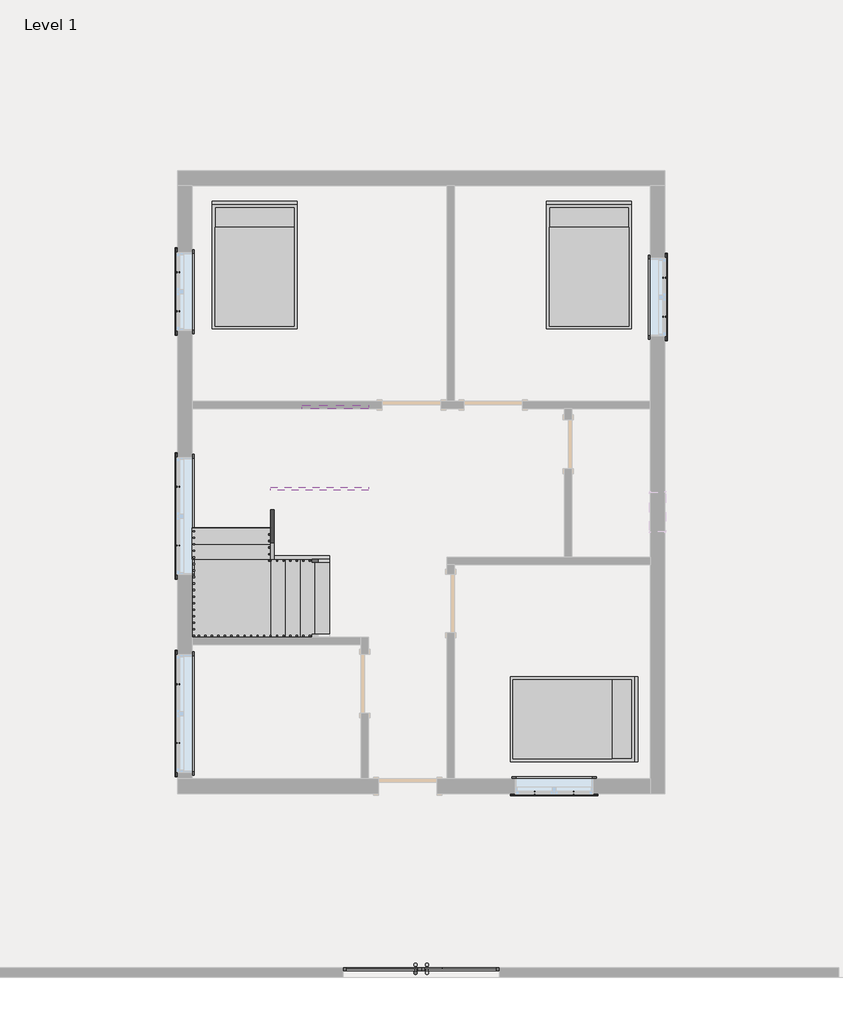
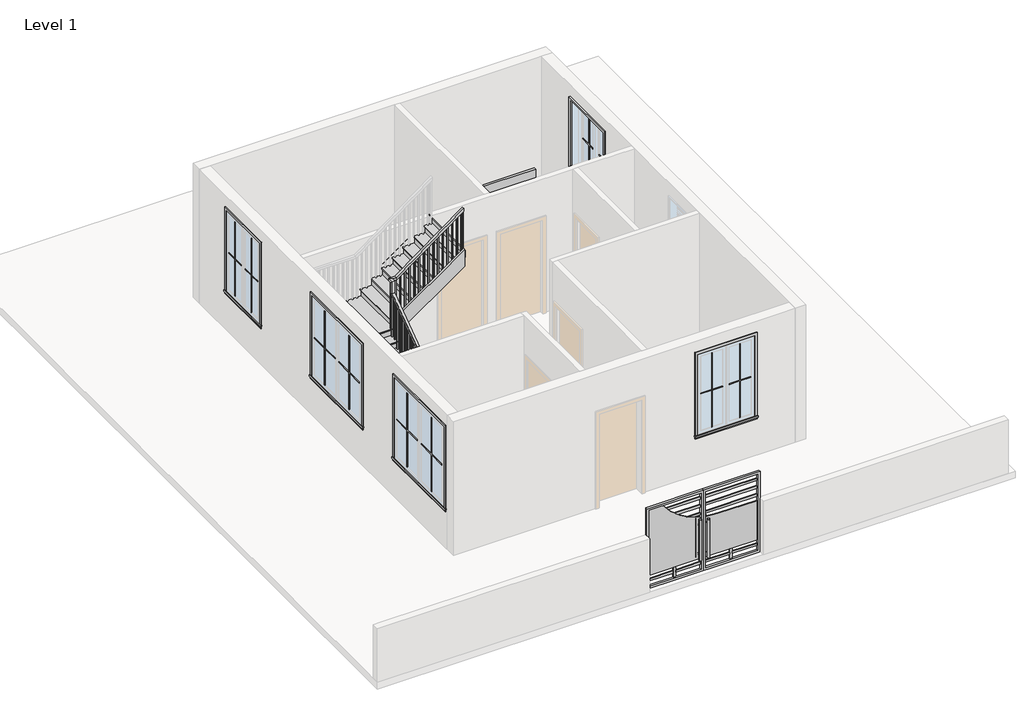
# One storey, part 3 of 3: 21 proxies, 5 members, 3 furniture elements, 1 railing, 1 stair flight.
"""IFC4 building model written with IfcOpenShell, lengths in millimetres."""

from ifc_helpers import new_model, si_unit, frame, origin, place, context, project, spatial, polyline, outline, extrude, faceted_brep, transform, mapped, element, save
from components import generic_models_113f6068, muntin_pattern_2x2_muntin_pattern_2x2_0a037076, muntin_pattern_2x2_muntin_pattern_2x2_e6f69628, muntin_pattern_2x2_muntin_pattern_2x2_2b4d9f72, muntin_pattern_2x2_muntin_pattern_2x2_ef995ed3, trim_window_exterior_flat_with_sill_b601e94a, trim_window_exterior_flat_with_sill_b7e4d11c, trim_window_interior_flat_picture_frame_bfefb25c, trim_window_interior_flat_picture_frame_936b8d2a, bed_17739_bed_17739_15c61121, stair_flight_0ad16ec4

model = new_model("IFC4")

# Units and contexts
model_context = context("Model", 3, world=origin())
ifc_project = project(units=[si_unit("LENGTHUNIT", "METRE", prefix="MILLI")], contexts=[model_context])

# Site, building, storey
site = spatial("IfcSite", under=ifc_project)
building = spatial("IfcBuilding", under=site)
storey = spatial("IfcBuildingStorey", under=building, Name="Level 1", Elevation=0.0)

# Proxies
placement = place(None, origin())
generic_models_shape = generic_models_113f6068(model_context)
element("IfcBuildingElementProxy", 1, Name="Generic Models", at=placement, inside=storey, context=model_context, shape_type="MappedRepresentation", body=[
    mapped(generic_models_shape, transform((-1254.3605391, -7873.6106437, 0.0), x_axis=(1.0, 0.0, 0.0), y_axis=(0.0, 1.0, 0.0), z_axis=(0.0, 0.0, 1.0))),
])
muntin_pattern_2x2_muntin_pattern_2x2_shape = muntin_pattern_2x2_muntin_pattern_2x2_0a037076(model_context)
element("IfcBuildingElementProxy", 2, Name="Muntin Pattern_2x2 : Muntin Pattern_2x2", ObjectType="Muntin Pattern_2x2 : Muntin Pattern_2x2", at=placement, inside=storey, context=model_context, shape_type="MappedRepresentation", body=[
    mapped(muntin_pattern_2x2_muntin_pattern_2x2_shape, transform((-5035.7855391, -4380.9248761, 984.25), x_axis=(0.0, 1.0, 0.0), y_axis=(-1.0, 0.0, 0.0), z_axis=(0.0, 0.0, 1.0))),
])
element("IfcBuildingElementProxy", 3, Name="Muntin Pattern_2x2 : Muntin Pattern_2x2", ObjectType="Muntin Pattern_2x2 : Muntin Pattern_2x2", at=placement, inside=storey, context=model_context, shape_type="MappedRepresentation", body=[
    mapped(muntin_pattern_2x2_muntin_pattern_2x2_shape, transform((-5035.7855391, -1310.6998761, 984.25), x_axis=(0.0, 1.0, 0.0), y_axis=(-1.0, 0.0, 0.0), z_axis=(0.0, 0.0, 1.0))),
])
muntin_pattern_2x2_muntin_pattern_2x2_2_shape = muntin_pattern_2x2_muntin_pattern_2x2_e6f69628(model_context)
element("IfcBuildingElementProxy", 4, Name="Muntin Pattern_2x2 : Muntin Pattern_2x2", ObjectType="Muntin Pattern_2x2 : Muntin Pattern_2x2", at=placement, inside=storey, context=model_context, shape_type="MappedRepresentation", body=[
    mapped(muntin_pattern_2x2_muntin_pattern_2x2_2_shape, transform((-5035.7855391, -3469.6998761, 984.25), x_axis=(0.0, -1.0, 0.0), y_axis=(1.0, 0.0, 0.0), z_axis=(0.0, 0.0, 1.0))),
])
element("IfcBuildingElementProxy", 5, Name="Muntin Pattern_2x2 : Muntin Pattern_2x2", ObjectType="Muntin Pattern_2x2 : Muntin Pattern_2x2", at=placement, inside=storey, context=model_context, shape_type="MappedRepresentation", body=[
    mapped(muntin_pattern_2x2_muntin_pattern_2x2_2_shape, transform((-5035.7855391, -399.4748761, 984.25), x_axis=(0.0, -1.0, 0.0), y_axis=(1.0, 0.0, 0.0), z_axis=(0.0, 0.0, 1.0))),
])
muntin_pattern_2x2_muntin_pattern_2x2_3_shape = muntin_pattern_2x2_muntin_pattern_2x2_2b4d9f72(model_context)
element("IfcBuildingElementProxy", 6, Name="Muntin Pattern_2x2 : Muntin Pattern_2x2", ObjectType="Muntin Pattern_2x2 : Muntin Pattern_2x2", at=placement, inside=storey, context=model_context, shape_type="MappedRepresentation", body=[
    mapped(muntin_pattern_2x2_muntin_pattern_2x2_3_shape, transform((1115.7769609, -5157.2123761, 984.25), x_axis=(-1.0, 0.0, 0.0), y_axis=(0.0, -1.0, 0.0), z_axis=(0.0, 0.0, 1.0))),
])
element("IfcBuildingElementProxy", 7, Name="Muntin Pattern_2x2 : Muntin Pattern_2x2", ObjectType="Muntin Pattern_2x2 : Muntin Pattern_2x2", at=placement, inside=storey, context=model_context, shape_type="MappedRepresentation", body=[
    mapped(muntin_pattern_2x2_muntin_pattern_2x2_3_shape, transform((2527.0644609, 2851.7251239, 984.25), x_axis=(0.0, -1.0, 0.0), y_axis=(1.0, 0.0, 0.0), z_axis=(0.0, 0.0, 1.0))),
])
element("IfcBuildingElementProxy", 8, Name="Muntin Pattern_2x2 : Muntin Pattern_2x2", ObjectType="Muntin Pattern_2x2 : Muntin Pattern_2x2", at=placement, inside=storey, context=model_context, shape_type="MappedRepresentation", body=[
    mapped(muntin_pattern_2x2_muntin_pattern_2x2_3_shape, transform((-5035.7855391, 2331.0251239, 984.25), x_axis=(0.0, 1.0, 0.0), y_axis=(-1.0, 0.0, 0.0), z_axis=(0.0, 0.0, 1.0))),
])
muntin_pattern_2x2_muntin_pattern_2x2_4_shape = muntin_pattern_2x2_muntin_pattern_2x2_ef995ed3(model_context)
element("IfcBuildingElementProxy", 9, Name="Muntin Pattern_2x2 : Muntin Pattern_2x2", ObjectType="Muntin Pattern_2x2 : Muntin Pattern_2x2", at=placement, inside=storey, context=model_context, shape_type="MappedRepresentation", body=[
    mapped(muntin_pattern_2x2_muntin_pattern_2x2_4_shape, transform((509.3519609, -5157.2123761, 984.25), x_axis=(1.0, 0.0, 0.0), y_axis=(0.0, 1.0, 0.0), z_axis=(0.0, 0.0, 1.0))),
])
element("IfcBuildingElementProxy", 10, Name="Muntin Pattern_2x2 : Muntin Pattern_2x2", ObjectType="Muntin Pattern_2x2 : Muntin Pattern_2x2", at=placement, inside=storey, context=model_context, shape_type="MappedRepresentation", body=[
    mapped(muntin_pattern_2x2_muntin_pattern_2x2_4_shape, transform((2527.0644609, 2245.3001239, 984.25), x_axis=(0.0, 1.0, 0.0), y_axis=(-1.0, 0.0, 0.0), z_axis=(0.0, 0.0, 1.0))),
])
element("IfcBuildingElementProxy", 11, Name="Muntin Pattern_2x2 : Muntin Pattern_2x2", ObjectType="Muntin Pattern_2x2 : Muntin Pattern_2x2", at=placement, inside=storey, context=model_context, shape_type="MappedRepresentation", body=[
    mapped(muntin_pattern_2x2_muntin_pattern_2x2_4_shape, transform((-5035.7855391, 2937.4501239, 984.25), x_axis=(0.0, -1.0, 0.0), y_axis=(1.0, 0.0, 0.0), z_axis=(0.0, 0.0, 1.0))),
])
trim_window_exterior_flat_with_sill_shape = trim_window_exterior_flat_with_sill_b601e94a(model_context)
element("IfcBuildingElementProxy", 12, Name="Trim-Window-Exterior-Flat : with Sill", ObjectType="Trim-Window-Exterior-Flat : with Sill", at=placement, inside=storey, context=model_context, shape_type="MappedRepresentation", body=[
    mapped(trim_window_exterior_flat_with_sill_shape, transform((-5045.3105391, -3925.3123761, 2743.2), x_axis=(0.0, -1.0, 0.0), y_axis=(0.0, 0.0, 1.0), z_axis=(-1.0, 0.0, 0.0))),
])
element("IfcBuildingElementProxy", 13, Name="Trim-Window-Exterior-Flat : with Sill", ObjectType="Trim-Window-Exterior-Flat : with Sill", at=placement, inside=storey, context=model_context, shape_type="MappedRepresentation", body=[
    mapped(trim_window_exterior_flat_with_sill_shape, transform((-5045.3105391, -855.0873761, 2743.2), x_axis=(0.0, -1.0, 0.0), y_axis=(0.0, 0.0, 1.0), z_axis=(-1.0, 0.0, 0.0))),
])
trim_window_exterior_flat_with_sill_2_shape = trim_window_exterior_flat_with_sill_b7e4d11c(model_context)
element("IfcBuildingElementProxy", 14, Name="Trim-Window-Exterior-Flat : with Sill", ObjectType="Trim-Window-Exterior-Flat : with Sill", at=placement, inside=storey, context=model_context, shape_type="MappedRepresentation", body=[
    mapped(trim_window_exterior_flat_with_sill_2_shape, transform((812.5644609, -5166.7373761, 2743.2), x_axis=(1.0, 0.0, 0.0), y_axis=(0.0, 0.0, 1.0), z_axis=(0.0, -1.0, 0.0))),
])
element("IfcBuildingElementProxy", 15, Name="Trim-Window-Exterior-Flat : with Sill", ObjectType="Trim-Window-Exterior-Flat : with Sill", at=placement, inside=storey, context=model_context, shape_type="MappedRepresentation", body=[
    mapped(trim_window_exterior_flat_with_sill_2_shape, transform((2536.5894609, 2548.5126239, 2743.2), x_axis=(0.0, 1.0, 0.0), y_axis=(0.0, 0.0, 1.0), z_axis=(1.0, 0.0, 0.0))),
])
element("IfcBuildingElementProxy", 16, Name="Trim-Window-Exterior-Flat : with Sill", ObjectType="Trim-Window-Exterior-Flat : with Sill", at=placement, inside=storey, context=model_context, shape_type="MappedRepresentation", body=[
    mapped(trim_window_exterior_flat_with_sill_2_shape, transform((-5045.3105391, 2634.2376239, 2743.2), x_axis=(0.0, -1.0, 0.0), y_axis=(0.0, 0.0, 1.0), z_axis=(-1.0, 0.0, 0.0))),
])
trim_window_interior_flat_picture_frame_shape = trim_window_interior_flat_picture_frame_bfefb25c(model_context)
element("IfcBuildingElementProxy", 17, Name="Trim-Window-Interior-Flat : Picture Frame", ObjectType="Trim-Window-Interior-Flat : Picture Frame", at=placement, inside=storey, context=model_context, shape_type="MappedRepresentation", body=[
    mapped(trim_window_interior_flat_picture_frame_shape, transform((-4816.7105391, -3925.3123761, 2743.2), x_axis=(0.0, 1.0, 0.0), y_axis=(0.0, 0.0, 1.0), z_axis=(1.0, 0.0, 0.0))),
])
element("IfcBuildingElementProxy", 18, Name="Trim-Window-Interior-Flat : Picture Frame", ObjectType="Trim-Window-Interior-Flat : Picture Frame", at=placement, inside=storey, context=model_context, shape_type="MappedRepresentation", body=[
    mapped(trim_window_interior_flat_picture_frame_shape, transform((-4816.7105391, -855.0873761, 2743.2), x_axis=(0.0, 1.0, 0.0), y_axis=(0.0, 0.0, 1.0), z_axis=(1.0, 0.0, 0.0))),
])
trim_window_interior_flat_picture_frame_2_shape = trim_window_interior_flat_picture_frame_936b8d2a(model_context)
element("IfcBuildingElementProxy", 19, Name="Trim-Window-Interior-Flat : Picture Frame", ObjectType="Trim-Window-Interior-Flat : Picture Frame", at=placement, inside=storey, context=model_context, shape_type="MappedRepresentation", body=[
    mapped(trim_window_interior_flat_picture_frame_2_shape, transform((812.5644609, -4938.1373761, 2743.2), x_axis=(-1.0, 0.0, 0.0), y_axis=(0.0, 0.0, 1.0), z_axis=(0.0, 1.0, 0.0))),
])
element("IfcBuildingElementProxy", 20, Name="Trim-Window-Interior-Flat : Picture Frame", ObjectType="Trim-Window-Interior-Flat : Picture Frame", at=placement, inside=storey, context=model_context, shape_type="MappedRepresentation", body=[
    mapped(trim_window_interior_flat_picture_frame_2_shape, transform((2307.9894609, 2548.5126239, 2743.2), x_axis=(0.0, -1.0, 0.0), y_axis=(0.0, 0.0, 1.0), z_axis=(-1.0, 0.0, 0.0))),
])
element("IfcBuildingElementProxy", 21, Name="Trim-Window-Interior-Flat : Picture Frame", ObjectType="Trim-Window-Interior-Flat : Picture Frame", at=placement, inside=storey, context=model_context, shape_type="MappedRepresentation", body=[
    mapped(trim_window_interior_flat_picture_frame_2_shape, transform((-4816.7105391, 2634.2376239, 2743.2), x_axis=(0.0, 1.0, 0.0), y_axis=(0.0, 0.0, 1.0), z_axis=(1.0, 0.0, 0.0))),
])

# Furniture
bed_17739_bed_17739_shape = bed_17739_bed_17739_15c61121(model_context)
element("IfcFurniture", 22, ObjectType="Bed_17739 : Bed_17739", at=placement, inside=storey, context=model_context, shape_type="MappedRepresentation", body=[
    mapped(bed_17739_bed_17739_shape, transform((-3845.1605391, 3024.7626239, 0.0), x_axis=(1.0, 0.0, 0.0), y_axis=(0.0, 1.0, 0.0), z_axis=(0.0, 0.0, 1.0))),
])
element("IfcFurniture", 23, ObjectType="Bed_17739 : Bed_17739", at=placement, inside=storey, context=model_context, shape_type="MappedRepresentation", body=[
    mapped(bed_17739_bed_17739_shape, transform((1355.4894609, 3024.7626239, 0.0), x_axis=(1.0, 0.0, 0.0), y_axis=(0.0, 1.0, 0.0), z_axis=(0.0, 0.0, 1.0))),
])
element("IfcFurniture", 24, ObjectType="Bed_17739 : Bed_17739", at=placement, inside=storey, context=model_context, shape_type="MappedRepresentation", body=[
    mapped(bed_17739_bed_17739_shape, transform((1101.4894609, -4011.0373761, 0.0), x_axis=(0.0, -1.0, 0.0), y_axis=(1.0, 0.0, 0.0), z_axis=(0.0, 0.0, 1.0))),
])

# Members
element("IfcMember", 25, ObjectType="Stringer - 2\" Width", at=placement, inside=storey, context=model_context, shape_type="SweptSolid", body=[
    extrude(outline(polyline([(0.0, -2683.1105391), (150.5087903, -2683.1105391), (150.5087903, -3112.2707489), (0.0, -2897.7957228), (0.0, -2683.1105391)])), frame((0.0, -2791.8373761, 0.0), z_axis=(0.0, 1.0, 0.0), x_axis=(0.0, 0.0, 1.0)), (0.0, 0.0, 1.0), 50.8),
])
element("IfcMember", 26, ObjectType="Stringer - 2\" Width", at=placement, inside=storey, context=model_context, shape_type="SweptSolid", body=[
    extrude(outline(polyline([(2327.4856495, -2580.7583047), (2683.4489938, -2073.5105391), (3055.8117181, -2073.5105391), (2327.4856495, -3111.3751869), (2327.4856495, -2580.7583047)])), frame((0.0, 814.9626239, 0.0), z_axis=(0.0, 1.0, 0.0), x_axis=(0.0, 0.0, 1.0)), (0.0, 0.0, 1.0), 50.8),
])
element("IfcMember", 27, ObjectType="Stringer - 2\" Width", at=placement, inside=storey, context=model_context, shape_type="SweptSolid", body=[
    extrude(outline(polyline([(0.0, -2683.1105391), (221.706455, -2683.1105391), (827.7415427, -3546.7105391), (455.3788184, -3546.7105391), (0.0, -2897.7957228), (0.0, -2683.1105391)])), frame((0.0, -1521.8373761, 0.0), z_axis=(0.0, 1.0, 0.0), x_axis=(0.0, 0.0, 1.0)), (0.0, 0.0, 1.0), 50.8),
])
element("IfcMember", 28, ObjectType="Stringer - 2\" Width", at=placement, inside=storey, context=model_context, shape_type="SweptSolid", body=[
    extrude(outline(polyline([(-1521.8373761, 650.3564629), (-1521.8373761, 1025.5327137), (-455.0373761, 1791.1786467), (-455.0373761, 1416.0023959), (-1521.8373761, 650.3564629)])), frame((-3597.5105391, 0.0, 0.0), z_axis=(1.0, 0.0, 0.0), x_axis=(0.0, 1.0, 0.0)), (0.0, 0.0, 1.0), 50.8),
])
element("IfcMember", 29, ObjectType="Stringer - 2\" Width", at=placement, inside=storey, context=model_context, shape_type="SweptSolid", body=[
    extrude(outline(polyline([(1986.3380339, -3597.5105391), (1613.9753096, -3597.5105391), (2683.4489938, -2073.5105391), (3055.8117181, -2073.5105391), (1986.3380339, -3597.5105391)])), frame((0.0, -455.0373761, 0.0), z_axis=(0.0, 1.0, 0.0), x_axis=(0.0, 0.0, 1.0)), (0.0, 0.0, 1.0), 50.8),
])

# Railing
element("IfcRailing", 30, ObjectType="Handrail - Rectangular", at=placement, inside=storey, context=model_context, shape_type="SolidModel", body=[
    faceted_brep([(-2683.1105391, -1572.6373761, 1074.8210526), (-2683.1105391, -1572.6373761, 1012.7605986), (-2683.1105391, -1521.8373761, 1012.7605986), (-2683.1105391, -1521.8373761, 1074.8210526), (-3521.3105391, -1572.6373761, 1663.0315789), (-3572.1105391, -1572.6373761, 1636.6202477), (-3572.1105391, -1521.8373761, 1636.6202477), (-3521.3105391, -1521.8373761, 1663.0315789), (-3521.3105391, -1572.6373761, 1931.615311), (-3572.1105391, -1572.6373761, 1880.815311), (-3572.1105391, -1521.8373761, 1880.815311), (-3521.3105391, -1521.8373761, 1931.615311), (-3648.3105391, -1572.6373761, 1931.615311), (-3648.3105391, -1572.6373761, 1880.815311), (-3597.5105391, -1521.8373761, 1880.815311), (-3597.5105391, -1521.8373761, 1931.615311), (-3648.3105391, -1445.6373761, 1931.615311), (-3648.3105391, -1429.2944467, 1880.815311), (-3597.5105391, -1429.2944467, 1880.815311), (-3597.5105391, -1445.6373761, 1931.615311), (-3648.3105391, -480.4373761, 2624.3425837), (-3648.3105391, -429.6373761, 2598.2725387), (-3597.5105391, -429.6373761, 2598.2725387), (-3597.5105391, -480.4373761, 2624.3425837), (-3648.3105391, -480.4373761, 2895.6), (-3648.3105391, -429.6373761, 2844.8), (-3597.5105391, -429.6373761, 2844.8), (-3597.5105391, -480.4373761, 2895.6), (-3648.3105391, -353.4373761, 2895.6), (-3648.3105391, -353.4373761, 2844.8), (-3597.5105391, -404.2373761, 2844.8), (-3597.5105391, -404.2373761, 2895.6), (-3521.3105391, -353.4373761, 2895.6), (-3504.6160355, -353.4373761, 2844.8), (-3504.6160355, -404.2373761, 2844.8), (-3521.3105391, -404.2373761, 2895.6), (-2073.5105391, -353.4373761, 3962.4), (-2073.5105391, -404.2373761, 3962.4), (-2073.5105391, -404.2373761, 3899.2987868), (-2073.5105391, -353.4373761, 3899.2987868)], [[[0, 1, 2, 3]], [[1, 0, 4, 5]], [[2, 1, 5, 6]], [[3, 2, 6, 7]], [[0, 3, 7, 4]], [[5, 4, 8, 9]], [[6, 5, 9, 10]], [[7, 6, 10, 11]], [[4, 7, 11, 8]], [[9, 8, 12, 13]], [[10, 9, 13, 14]], [[11, 10, 14, 15]], [[8, 11, 15, 12]], [[13, 12, 16, 17]], [[14, 13, 17, 18]], [[15, 14, 18, 19]], [[12, 15, 19, 16]], [[17, 16, 20, 21]], [[18, 17, 21, 22]], [[19, 18, 22, 23]], [[16, 19, 23, 20]], [[21, 20, 24, 25]], [[22, 21, 25, 26]], [[23, 22, 26, 27]], [[20, 23, 27, 24]], [[25, 24, 28, 29]], [[26, 25, 29, 30]], [[27, 26, 30, 31]], [[24, 27, 31, 28]], [[29, 28, 32, 33]], [[30, 29, 33, 34]], [[31, 30, 34, 35]], [[28, 31, 35, 32]], [[36, 37, 38, 39]], [[33, 32, 36, 39]], [[34, 33, 39, 38]], [[35, 34, 38, 37]], [[32, 35, 37, 36]]]),
    extrude(outline(polyline([(3887.6014184, -2089.3855391), (3873.5645763, -2108.4355391), (2887.5789474, -2108.4355391), (2887.5789474, -2089.3855391), (3887.6014184, -2089.3855391)])), frame((0.0, -388.3623761, 0.0), z_axis=(0.0, 1.0, 0.0), x_axis=(0.0, 0.0, 1.0)), (0.0, 0.0, 1.0), 19.05),
    extrude(outline(polyline([(3812.7382605, -2190.9855391), (3798.7014184, -2210.0355391), (2887.5789474, -2210.0355391), (2887.5789474, -2190.9855391), (3812.7382605, -2190.9855391)])), frame((0.0, -388.3623761, 0.0), z_axis=(0.0, 1.0, 0.0), x_axis=(0.0, 0.0, 1.0)), (0.0, 0.0, 1.0), 19.05),
    extrude(outline(polyline([(3737.8751026, -2292.5855391), (3723.8382605, -2311.6355391), (2727.1578947, -2311.6355391), (2727.1578947, -2292.5855391), (3737.8751026, -2292.5855391)])), frame((0.0, -388.3623761, 0.0), z_axis=(0.0, 1.0, 0.0), x_axis=(0.0, 0.0, 1.0)), (0.0, 0.0, 1.0), 19.05),
    extrude(outline(polyline([(3663.0119447, -2394.1855391), (3648.9751026, -2413.2355391), (2727.1578947, -2413.2355391), (2727.1578947, -2394.1855391), (3663.0119447, -2394.1855391)])), frame((0.0, -388.3623761, 0.0), z_axis=(0.0, 1.0, 0.0), x_axis=(0.0, 0.0, 1.0)), (0.0, 0.0, 1.0), 19.05),
    extrude(outline(polyline([(3588.1487868, -2495.7855391), (3574.1119447, -2514.8355391), (2566.7368421, -2514.8355391), (2566.7368421, -2495.7855391), (3588.1487868, -2495.7855391)])), frame((0.0, -388.3623761, 0.0), z_axis=(0.0, 1.0, 0.0), x_axis=(0.0, 0.0, 1.0)), (0.0, 0.0, 1.0), 19.05),
    extrude(outline(polyline([(3513.2856289, -2597.3855391), (3499.2487868, -2616.4355391), (2566.7368421, -2616.4355391), (2566.7368421, -2597.3855391), (3513.2856289, -2597.3855391)])), frame((0.0, -388.3623761, 0.0), z_axis=(0.0, 1.0, 0.0), x_axis=(0.0, 0.0, 1.0)), (0.0, 0.0, 1.0), 19.05),
    extrude(outline(polyline([(3438.422471, -2698.9855391), (3424.3856289, -2718.0355391), (2406.3157895, -2718.0355391), (2406.3157895, -2698.9855391), (3438.422471, -2698.9855391)])), frame((0.0, -388.3623761, 0.0), z_axis=(0.0, 1.0, 0.0), x_axis=(0.0, 0.0, 1.0)), (0.0, 0.0, 1.0), 19.05),
    extrude(outline(polyline([(3363.5593132, -2800.5855391), (3349.522471, -2819.6355391), (2406.3157895, -2819.6355391), (2406.3157895, -2800.5855391), (3363.5593132, -2800.5855391)])), frame((0.0, -388.3623761, 0.0), z_axis=(0.0, 1.0, 0.0), x_axis=(0.0, 0.0, 1.0)), (0.0, 0.0, 1.0), 19.05),
    extrude(outline(polyline([(3288.6961553, -2902.1855391), (3274.6593132, -2921.2355391), (2406.3157895, -2921.2355391), (2406.3157895, -2902.1855391), (3288.6961553, -2902.1855391)])), frame((0.0, -388.3623761, 0.0), z_axis=(0.0, 1.0, 0.0), x_axis=(0.0, 0.0, 1.0)), (0.0, 0.0, 1.0), 19.05),
    extrude(outline(polyline([(3213.8329974, -3003.7855391), (3199.7961553, -3022.8355391), (2245.8947368, -3022.8355391), (2245.8947368, -3003.7855391), (3213.8329974, -3003.7855391)])), frame((0.0, -388.3623761, 0.0), z_axis=(0.0, 1.0, 0.0), x_axis=(0.0, 0.0, 1.0)), (0.0, 0.0, 1.0), 19.05),
    extrude(outline(polyline([(3138.9698395, -3105.3855391), (3124.9329974, -3124.4355391), (2245.8947368, -3124.4355391), (2245.8947368, -3105.3855391), (3138.9698395, -3105.3855391)])), frame((0.0, -388.3623761, 0.0), z_axis=(0.0, 1.0, 0.0), x_axis=(0.0, 0.0, 1.0)), (0.0, 0.0, 1.0), 19.05),
    extrude(outline(polyline([(3064.1066816, -3206.9855391), (3050.0698395, -3226.0355391), (2085.4736842, -3226.0355391), (2085.4736842, -3206.9855391), (3064.1066816, -3206.9855391)])), frame((0.0, -388.3623761, 0.0), z_axis=(0.0, 1.0, 0.0), x_axis=(0.0, 0.0, 1.0)), (0.0, 0.0, 1.0), 19.05),
    extrude(outline(polyline([(2989.2435237, -3308.5855391), (2975.2066816, -3327.6355391), (2085.4736842, -3327.6355391), (2085.4736842, -3308.5855391), (2989.2435237, -3308.5855391)])), frame((0.0, -388.3623761, 0.0), z_axis=(0.0, 1.0, 0.0), x_axis=(0.0, 0.0, 1.0)), (0.0, 0.0, 1.0), 19.05),
    extrude(outline(polyline([(2914.3803658, -3410.1855391), (2900.3435237, -3429.2355391), (1925.0526316, -3429.2355391), (1925.0526316, -3410.1855391), (2914.3803658, -3410.1855391)])), frame((0.0, -388.3623761, 0.0), z_axis=(0.0, 1.0, 0.0), x_axis=(0.0, 0.0, 1.0)), (0.0, 0.0, 1.0), 19.05),
    extrude(outline(polyline([(2839.5172079, -3511.7855391), (2825.4803658, -3530.8355391), (1925.0526316, -3530.8355391), (1925.0526316, -3511.7855391), (2839.5172079, -3511.7855391)])), frame((0.0, -388.3623761, 0.0), z_axis=(0.0, 1.0, 0.0), x_axis=(0.0, 0.0, 1.0)), (0.0, 0.0, 1.0), 19.05),
    extrude(outline(polyline([(-3613.3855391, -439.1623761), (-3632.4355391, -439.1623761), (-3632.4355391, -420.1123761), (-3613.3855391, -420.1123761), (-3613.3855391, -439.1623761)])), frame((0.0, 0.0, 1604.2105263), z_axis=(0.0, 0.0, 1.0), x_axis=(1.0, 0.0, 0.0)), (0.0, 0.0, 1.0), 1240.5894737),
    extrude(outline(polyline([(-540.7623761, 2518.5177541), (-521.7123761, 2532.1900029), (-521.7123761, 1604.2105263), (-540.7623761, 1604.2105263), (-540.7623761, 2518.5177541)])), frame((-3632.4355391, 0.0, 0.0), z_axis=(1.0, 0.0, 0.0), x_axis=(0.0, 1.0, 0.0)), (0.0, 0.0, 1.0), 19.05),
    extrude(outline(polyline([(-642.3623761, 2445.5990938), (-623.3123761, 2459.2713426), (-623.3123761, 1443.7894737), (-642.3623761, 1443.7894737), (-642.3623761, 2445.5990938)])), frame((-3632.4355391, 0.0, 0.0), z_axis=(1.0, 0.0, 0.0), x_axis=(0.0, 1.0, 0.0)), (0.0, 0.0, 1.0), 19.05),
    extrude(outline(polyline([(-743.9623761, 2372.6804335), (-724.9123761, 2386.3526823), (-724.9123761, 1443.7894737), (-743.9623761, 1443.7894737), (-743.9623761, 2372.6804335)])), frame((-3632.4355391, 0.0, 0.0), z_axis=(1.0, 0.0, 0.0), x_axis=(0.0, 1.0, 0.0)), (0.0, 0.0, 1.0), 19.05),
    extrude(outline(polyline([(-845.5623761, 2299.7617732), (-826.5123761, 2313.434022), (-826.5123761, 1443.7894737), (-845.5623761, 1443.7894737), (-845.5623761, 2299.7617732)])), frame((-3632.4355391, 0.0, 0.0), z_axis=(1.0, 0.0, 0.0), x_axis=(0.0, 1.0, 0.0)), (0.0, 0.0, 1.0), 19.05),
    extrude(outline(polyline([(-947.1623761, 2226.8431129), (-928.1123761, 2240.5153617), (-928.1123761, 1283.3684211), (-947.1623761, 1283.3684211), (-947.1623761, 2226.8431129)])), frame((-3632.4355391, 0.0, 0.0), z_axis=(1.0, 0.0, 0.0), x_axis=(0.0, 1.0, 0.0)), (0.0, 0.0, 1.0), 19.05),
    extrude(outline(polyline([(-1048.7623761, 2153.9244526), (-1029.7123761, 2167.5967014), (-1029.7123761, 1283.3684211), (-1048.7623761, 1283.3684211), (-1048.7623761, 2153.9244526)])), frame((-3632.4355391, 0.0, 0.0), z_axis=(1.0, 0.0, 0.0), x_axis=(0.0, 1.0, 0.0)), (0.0, 0.0, 1.0), 19.05),
    extrude(outline(polyline([(-1150.3623761, 2081.0057923), (-1131.3123761, 2094.6780411), (-1131.3123761, 1122.9473684), (-1150.3623761, 1122.9473684), (-1150.3623761, 2081.0057923)])), frame((-3632.4355391, 0.0, 0.0), z_axis=(1.0, 0.0, 0.0), x_axis=(0.0, 1.0, 0.0)), (0.0, 0.0, 1.0), 19.05),
    extrude(outline(polyline([(-1251.9623761, 2008.087132), (-1232.9123761, 2021.7593808), (-1232.9123761, 1122.9473684), (-1251.9623761, 1122.9473684), (-1251.9623761, 2008.087132)])), frame((-3632.4355391, 0.0, 0.0), z_axis=(1.0, 0.0, 0.0), x_axis=(0.0, 1.0, 0.0)), (0.0, 0.0, 1.0), 19.05),
    extrude(outline(polyline([(-1353.5623761, 1935.1684718), (-1334.5123761, 1948.8407206), (-1334.5123761, 962.5263158), (-1353.5623761, 962.5263158), (-1353.5623761, 1935.1684718)])), frame((-3632.4355391, 0.0, 0.0), z_axis=(1.0, 0.0, 0.0), x_axis=(0.0, 1.0, 0.0)), (0.0, 0.0, 1.0), 19.05),
    extrude(outline(polyline([(-1455.1623761, 1862.2498115), (-1436.1123761, 1875.9220603), (-1436.1123761, 962.5263158), (-1455.1623761, 962.5263158), (-1455.1623761, 1862.2498115)])), frame((-3632.4355391, 0.0, 0.0), z_axis=(1.0, 0.0, 0.0), x_axis=(0.0, 1.0, 0.0)), (0.0, 0.0, 1.0), 19.05),
    extrude(outline(polyline([(-3587.9855391, -1537.7123761), (-3587.9855391, -1556.7623761), (-3607.0355391, -1556.7623761), (-3607.0355391, -1537.7123761), (-3587.9855391, -1537.7123761)])), frame((0.0, 0.0, 802.1052632), z_axis=(0.0, 0.0, 1.0), x_axis=(1.0, 0.0, 0.0)), (0.0, 0.0, 1.0), 1078.7100478),
    extrude(outline(polyline([(1576.462353, -3486.3855391), (1589.830774, -3505.4355391), (641.6842105, -3505.4355391), (641.6842105, -3486.3855391), (1576.462353, -3486.3855391)])), frame((0.0, -1556.7623761, 0.0), z_axis=(0.0, 1.0, 0.0), x_axis=(0.0, 0.0, 1.0)), (0.0, 0.0, 1.0), 19.05),
    extrude(outline(polyline([(1505.1641074, -3384.7855391), (1518.5325284, -3403.8355391), (641.6842105, -3403.8355391), (641.6842105, -3384.7855391), (1505.1641074, -3384.7855391)])), frame((0.0, -1556.7623761, 0.0), z_axis=(0.0, 1.0, 0.0), x_axis=(0.0, 0.0, 1.0)), (0.0, 0.0, 1.0), 19.05),
    extrude(outline(polyline([(1433.8658617, -3283.1855391), (1447.2342828, -3302.2355391), (481.2631579, -3302.2355391), (481.2631579, -3283.1855391), (1433.8658617, -3283.1855391)])), frame((0.0, -1556.7623761, 0.0), z_axis=(0.0, 1.0, 0.0), x_axis=(0.0, 0.0, 1.0)), (0.0, 0.0, 1.0), 19.05),
    extrude(outline(polyline([(1362.5676161, -3181.5855391), (1375.9360372, -3200.6355391), (481.2631579, -3200.6355391), (481.2631579, -3181.5855391), (1362.5676161, -3181.5855391)])), frame((0.0, -1556.7623761, 0.0), z_axis=(0.0, 1.0, 0.0), x_axis=(0.0, 0.0, 1.0)), (0.0, 0.0, 1.0), 19.05),
    extrude(outline(polyline([(1291.2693705, -3079.9855391), (1304.6377916, -3099.0355391), (320.8421053, -3099.0355391), (320.8421053, -3079.9855391), (1291.2693705, -3079.9855391)])), frame((0.0, -1556.7623761, 0.0), z_axis=(0.0, 1.0, 0.0), x_axis=(0.0, 0.0, 1.0)), (0.0, 0.0, 1.0), 19.05),
    extrude(outline(polyline([(1219.9711249, -2978.3855391), (1233.3395459, -2997.4355391), (320.8421053, -2997.4355391), (320.8421053, -2978.3855391), (1219.9711249, -2978.3855391)])), frame((0.0, -1556.7623761, 0.0), z_axis=(0.0, 1.0, 0.0), x_axis=(0.0, 0.0, 1.0)), (0.0, 0.0, 1.0), 19.05),
    extrude(outline(polyline([(1148.6728793, -2876.7855391), (1162.0413003, -2895.8355391), (160.4210526, -2895.8355391), (160.4210526, -2876.7855391), (1148.6728793, -2876.7855391)])), frame((0.0, -1556.7623761, 0.0), z_axis=(0.0, 1.0, 0.0), x_axis=(0.0, 0.0, 1.0)), (0.0, 0.0, 1.0), 19.05),
    extrude(outline(polyline([(1077.3746337, -2775.1855391), (1090.7430547, -2794.2355391), (160.4210526, -2794.2355391), (160.4210526, -2775.1855391), (1077.3746337, -2775.1855391)])), frame((0.0, -1556.7623761, 0.0), z_axis=(0.0, 1.0, 0.0), x_axis=(0.0, 0.0, 1.0)), (0.0, 0.0, 1.0), 19.05),
    extrude(outline(polyline([(-3613.3855391, -388.3623761), (-3632.4355391, -388.3623761), (-3632.4355391, -369.3123761), (-3613.3855391, -369.3123761), (-3613.3855391, -388.3623761)])), frame((0.0, 0.0, 1764.6315789), z_axis=(0.0, 0.0, 1.0), x_axis=(1.0, 0.0, 0.0)), (0.0, 0.0, 1.0), 1080.1684211),
    extrude(outline(polyline([(-3613.3855391, -1537.7123761), (-3613.3855391, -1556.7623761), (-3632.4355391, -1556.7623761), (-3632.4355391, -1537.7123761), (-3613.3855391, -1537.7123761)])), frame((0.0, 0.0, 802.1052632), z_axis=(0.0, 0.0, 1.0), x_axis=(1.0, 0.0, 0.0)), (0.0, 0.0, 1.0), 1078.7100478),
    extrude(outline(polyline([(3899.2987868, -2073.5105391), (3885.2619447, -2092.5605391), (2887.5789474, -2092.5605391), (2887.5789474, -2073.5105391), (3899.2987868, -2073.5105391)])), frame((0.0, -388.3623761, 0.0), z_axis=(0.0, 1.0, 0.0), x_axis=(0.0, 0.0, 1.0)), (0.0, 0.0, 1.0), 19.05),
    extrude(outline(polyline([(1012.7605986, -2683.1105391), (1026.1290196, -2702.1605391), (160.4210526, -2702.1605391), (160.4210526, -2683.1105391), (1012.7605986, -2683.1105391)])), frame((0.0, -1556.7623761, 0.0), z_axis=(0.0, 1.0, 0.0), x_axis=(0.0, 0.0, 1.0)), (0.0, 0.0, 1.0), 19.05),
])

# Stair flight
stair_flight_shape = stair_flight_0ad16ec4(model_context)
element("IfcStairFlight", 31, ObjectType="2\" Tread 1\" Nosing 1/4\" Riser", at=placement, inside=storey, context=model_context, shape_type="MappedRepresentation", body=[
    mapped(stair_flight_shape, transform((0.0, 0.0, 0.0), x_axis=(1.0, 0.0, 0.0), y_axis=(0.0, 1.0, 0.0), z_axis=(0.0, 0.0, 1.0))),
])

save(model, "model.ifc")

# Revit data of these elements
# Type
#   sheet = none
#   pipe = none
#   handal = none
#   faram = none
#   Default Elevation = 0
# Type "Muntin Pattern_2x2 : Muntin Pattern_2x2"
#   Width [instance default] = 4' - 0"
#   Thickness = 0' - 0 1/2"
#   Height [instance default] = 4' - 0"
#   Distance = 0' - 0 3/4"
#   Interior Material [instance default] = none
#   Exterior Material [instance default] = none
#   Default Elevation = 0
# Type "Trim-Window-Exterior-Flat : with Sill"
#   Trim Width = 0' - 2 1/4"
#   Trim Thickness_Picture Frame = 0' - 1 1/4"
#   Trim Thickness_with Sill = 0' - 0 3/4"
#   Sill Thickness = 0' - 1 1/4"
#   Opening Width [instance default] = 2' - 0"
#   Opening Height [instance default] = 3' - 0"
#   Default Elevation = 4' - 0"
#   Sill = yes
#   Picture Frame = no
#   Trim Material [instance default] = none
# Type "Trim-Window-Interior-Flat : Picture Frame"
#   Trim Thickness_Picture Frame = 0' - 1 1/4"
#   Trim Width = 0' - 2 1/4"
#   Trim Thickness_with Sill = 0' - 0 3/4"
#   Sill Thickness = 0' - 1 1/4"
#   Opening Width [instance default] = 2' - 0"
#   Opening Height [instance default] = 3' - 0"
#   Default Elevation = 4' - 0"
#   Sill = no
#   Picture Frame = yes
#   Trim Material [instance default] = none
# Type "Bed_17739 : Bed_17739"
#   Default Elevation = 0
# Type "Handrail - Rectangular"
#   Assembly Code = "C2010400"
#   built-in parameter 1008612 = 0.0416667 (stored number, unit not read)
#   built-in parameter 1008611 = 0.0416667 (stored number, unit not read)
#   built-in parameter 1008609 = 0.333333 (stored number, unit not read)
#   built-in parameter 1008604 = 0.166667 (stored number, unit not read)
#   built-in parameter 1008603 = 0.166667 (stored number, unit not read)
#   Railing Height = 3' - 0"
#   built-in parameter 1008630 = 2
#   built-in parameter 1008610 = 2
#   built-in parameter 1008618 = Baluster - Square : 3/4"
# Element 1 (IfcBuildingElementProxy)
#   Phase Created = New Construction
# Elements 2, 3, 4, 5 (IfcBuildingElementProxy, "Muntin Pattern_2x2 : Muntin Pattern_2x2")
#   Width = 2' - 6 5/8"
#   Height = 5' - 6 1/2"
#   Interior Material = Wood - Stained
#   Exterior Material = Clad - White
#   Phase Created = New Construction
#   Materials on its faces: "Clad - White", "Wood - Stained"
# Elements 6, 7, 8, 9, 10, 11 (IfcBuildingElementProxy, "Muntin Pattern_2x2 : Muntin Pattern_2x2")
#   Width = 1' - 6 5/8"
#   Height = 5' - 6 1/2"
#   Interior Material = Wood - Stained
#   Exterior Material = Clad - White
#   Phase Created = New Construction
#   Materials on its faces: "Clad - White", "Wood - Stained"
# Elements 12, 13 (IfcBuildingElementProxy, "Trim-Window-Exterior-Flat : with Sill")
#   Opening Width = 6' - 0"
#   Opening Height = 6' - 0"
#   Trim Material = Clad - White
#   Phase Created = New Construction
#   Materials on its faces: "Clad - White"
# Elements 14, 15, 16 (IfcBuildingElementProxy, "Trim-Window-Exterior-Flat : with Sill")
#   Opening Width = 4' - 0"
#   Opening Height = 6' - 0"
#   Trim Material = Clad - White
#   Phase Created = New Construction
#   Materials on its faces: "Clad - White"
# Elements 17, 18 (IfcBuildingElementProxy, "Trim-Window-Interior-Flat : Picture Frame")
#   Opening Width = 6' - 0"
#   Opening Height = 6' - 0"
#   Trim Material = Wood - Stained
#   Phase Created = New Construction
#   Materials on its faces: "Wood - Stained"
# Elements 19, 20, 21 (IfcBuildingElementProxy, "Trim-Window-Interior-Flat : Picture Frame")
#   Opening Width = 4' - 0"
#   Opening Height = 6' - 0"
#   Trim Material = Wood - Stained
#   Phase Created = New Construction
#   Materials on its faces: "Wood - Stained"
# Elements 22, 23, 24 (IfcFurniture, "Bed_17739 : Bed_17739")
#   Phase Created = New Construction
#   Materials on its faces: "legs", "sheets", "bed frame", "Blanket"
# Elements 25, 26, 27, 28, 29 (IfcMember, "Stringer - 2\" Width")
#   Phase Created = New Construction
# Element 30 (IfcRailing, "Handrail - Rectangular")
#   Phase Created = New Construction
# Element 31 (IfcStairFlight, "2\" Tread 1\" Nosing 1/4\" Riser")
#   Phase Created = New Construction
# Materials
#   "Clad - White": class "Wood", colour RGB 242 242 238, transparency 0, Cost = 0
#   "Wood - Stained": class "Wood", colour RGB 224 178 126, transparency 0, Cost = 0
#   "legs": colour RGB 90 73 37, transparency 0, Cost = 0
#   "sheets": colour RGB 200 195 176, transparency 0, Cost = 0
#   "bed frame": colour RGB 90 73 37, transparency 0, Cost = 0
#   "Blanket": class "System", colour RGB 59 0 1, transparency 0, Cost = 0
